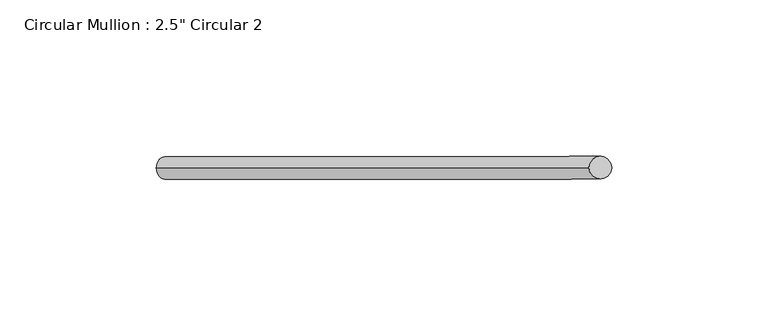
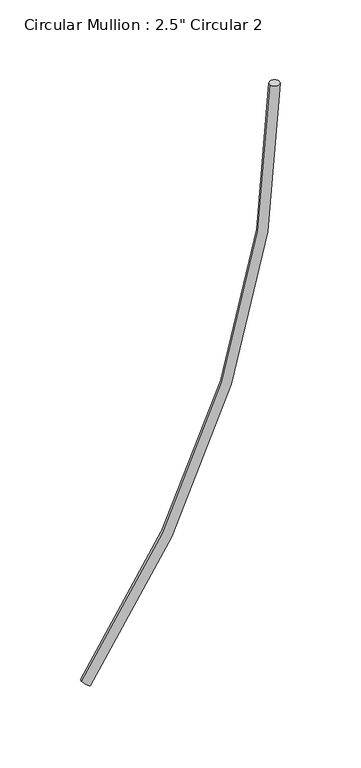
"""IFC4 building model written with IfcOpenShell, lengths in millimetres: member geometry."""

from ifc_helpers import new_model, si_unit, point, frame, origin, place, context, project, spatial, circle_curve, ellipse_curve, trimmed, source, transform, mapped, element, save
from ifc_brep_helpers import plane_surface, revolved_surface, advanced_brep


def member_a55882dd(model_context):
    return source(origin(), model_context, "Body", "AdvancedBrep", [
        advanced_brep(
        [(-145.4912, 0.0, -414.7566), (-7.239, 0.0, 0.0), (0.0, 0.0, 0.0), (-139.7, 0.0, -419.1)],
        [
            (0, 1, circle_curve(frame((-698.5, 0.0, 0.0), z_axis=(0.0, -1.0, 0.0), x_axis=(1.0, 0.0, 0.0)), 691.261)),
            (1, 2, circle_curve(frame((-3.6195, 0.0, 0.0), z_axis=(0.0, 0.0, -1.0), x_axis=(1.0, 0.0, 0.0)), 3.6195)),
            (2, 3, circle_curve(frame((-698.5, 0.0, 0.0), z_axis=(0.0, 1.0, 0.0), x_axis=(1.0, 0.0, 0.0)), 698.5)),
            (3, 0, circle_curve(frame((-142.5956, 0.0, -416.9283), z_axis=(0.599999999999985, 0.0, 0.8000000000000113), x_axis=(0.8000000000000113, 0.0, -0.599999999999985)), 3.6195)),
            (2, 1, circle_curve(frame((-3.6195, 0.0, 0.0), z_axis=(0.0, 0.0, -1.0), x_axis=(1.0, 0.0, 0.0)), 3.6195)),
            (0, 3, circle_curve(frame((-142.5956, 0.0, -416.9283), z_axis=(0.5999999999999851, 0.0, 0.8000000000000111), x_axis=(0.8000000000000111, 0.0, -0.5999999999999851)), 3.6195)),
        ],
        [
            revolved_surface(trimmed(ellipse_curve(frame((-3.6195, 0.0, 0.0), z_axis=(0.0, 0.0, 1.0), x_axis=(1.0, 0.0, 0.0)), 3.6195, 3.6195), [point((0.0, 0.0, 0.0))], [point((-7.239, 0.0, 0.0))], True, "CARTESIAN"), (-698.5, 0.0, 0.0), (0.0, 1.0, 0.0)),
            revolved_surface(trimmed(ellipse_curve(frame((-3.6195, 0.0, 0.0), z_axis=(0.0, 0.0, 1.0), x_axis=(1.0, 0.0, 0.0)), 3.6195, 3.6195), [point((-7.239, 0.0, 0.0))], [point((0.0, 0.0, 0.0))], True, "CARTESIAN"), (-698.5, 0.0, 0.0), (0.0, 1.0, 0.0)),
            plane_surface(frame((-304.8, 0.0, 0.0), z_axis=(0.0, 0.0, 1.0), x_axis=(0.0, 1.0, 0.0))),
            plane_surface(frame((104.14, 0.0, -601.98), z_axis=(-0.5999999999999851, 0.0, -0.8000000000000113), x_axis=(0.0, -1.0, 0.0))),
        ],
        [
            (0, [[1, 2, 3, 4]]),
            (1, [[-3, 5, -1, 6]]),
            (2, [[-2, -5]]),
            (3, [[-6, -4]]),
        ],
    ),
    ])


if __name__ == "__main__":
    model = new_model("IFC4")
    model_context = context("Model", 3, world=origin())
    ifc_project = project(units=[si_unit("LENGTHUNIT", "METRE", prefix="MILLI")], contexts=[model_context])
    site = spatial("IfcSite", under=ifc_project)
    building = spatial("IfcBuilding", under=site)
    placement = place(None, origin())
    member_shape = member_a55882dd(model_context)
    element("IfcMember", 1, ObjectType="Circular Mullion : 2.5\" Circular 2", at=placement, inside=building, context=model_context, shape_type="MappedRepresentation", body=[
        mapped(member_shape, transform((0.0, 0.0, 0.0), x_axis=(1.0, 0.0, 0.0), y_axis=(0.0, 1.0, 0.0), z_axis=(0.0, 0.0, 1.0))),
    ])
    save(model, "model.ifc")

# Revit data of these elements
# Type "Circular Mullion : 2.5\" Circular 2"
#   built-in parameter 1007350 = 0.011875 (stored number, unit not read)
# Element 1 (IfcMember, "Circular Mullion : 2.5\" Circular 2")
#   Materials on its faces: "Aluminum"
# Materials
#   "Aluminum": class "Metal", colour RGB 247 247 247, transparency 0, Description = "Aluminum 6061", Cost = 0
